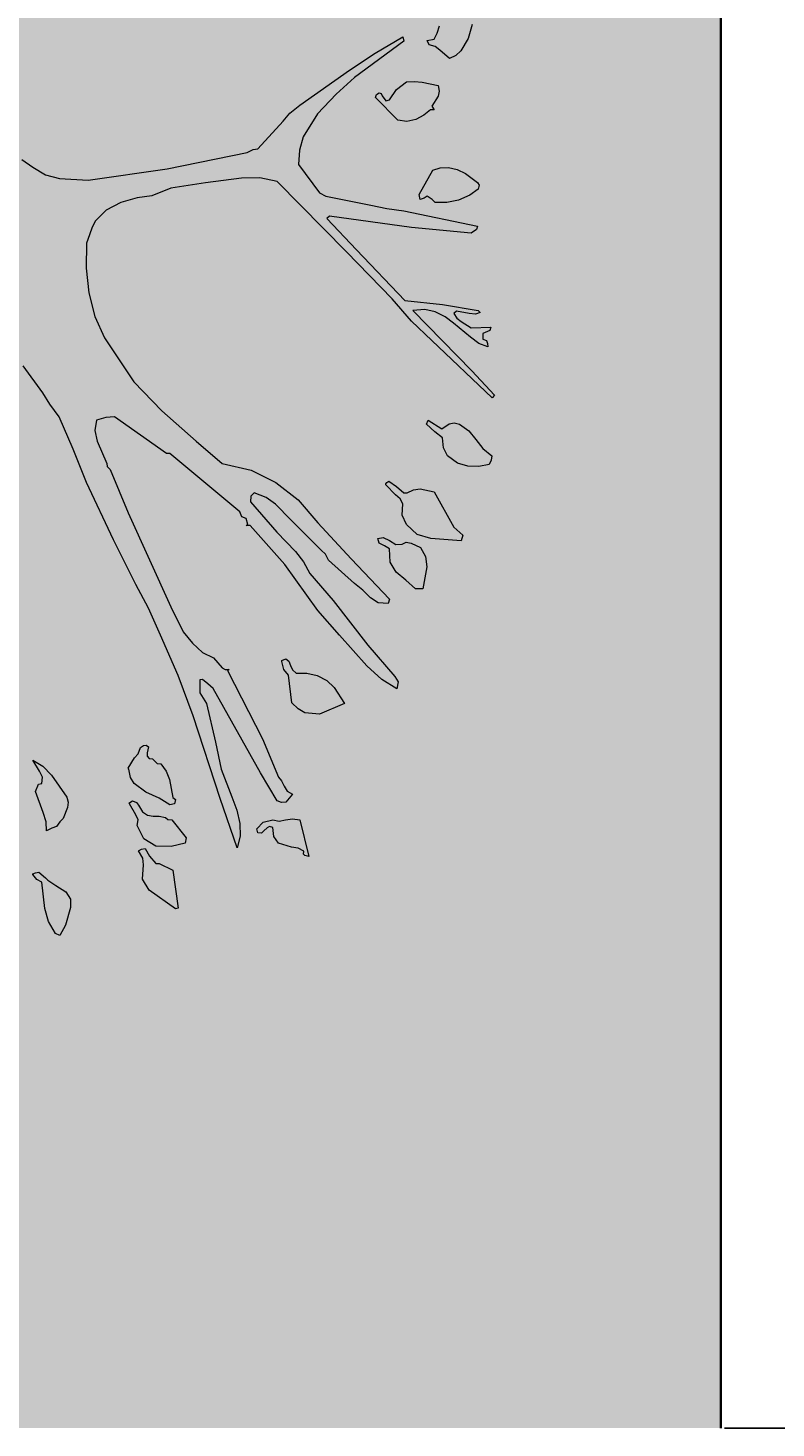
# Model space of a CAD drawing. Units: inches. Extents: x 84 to 1044, y -280 to 906.
# Tile 88 of 105: x 883 to 897, y 400 to 426. Entities that reach past the tile are written whole.
import ezdxf

# ---------------------------------------------------------------- set-up
doc = ezdxf.new("R2010")
doc.units = ezdxf.units.IN
for name, color, linetype, lineweight in [('A-ANNO-DIMS', 2, 'Continuous', 18), ('L-PLNT', 114, 'Continuous', 15), ('WALL', 250, 'Continuous', 35)]:
    doc.layers.add(name, color=color, linetype=linetype, lineweight=lineweight)
doc.layers.add('L-PLNT-PATT', color=9, linetype='Continuous', lineweight=9, true_color=0xafd9aa)
doc.styles.get("Standard").update_dxf_attribs({"font": 'arial.ttf'})
doc.dimstyles.get("Standard").update_dxf_attribs({"dimtxt": 0.18, "dimasz": 0.18, "dimexe": 0.18, "dimexo": 0.0625, "dimgap": 0.09, "dimtad": 0, "dimtih": 1, "dimtoh": 1, "dimdec": 4, "dimzin": 0, "dimdsep": 46, "dimtxsty": 'Standard', "dimcen": 0.09, "dimadec": 0, "dimazin": 0, "dimtfac": 1, "dimtdec": 4, "dimtofl": 0, "dimtmove": 0, "dimatfit": 3, "dimfxl": 1, "dimtolj": 1, "dimtzin": 0, "dimarcsym": 0})

# ---------------------------------------------------------------- blocks, each defined once
blk = doc.blocks.new('A$C37E508DF')
for p, q in [((1.3421, 1.0861), (1.3455, 1.0934)), ((1.3455, 1.0934), (1.3485, 1.102)), ((1.3875, 1.1037), (1.3828, 1.087)), ((1.3057, 1.0835), (1.2469, 1.0402)), ((1.2713, 1.0694), (1.3044, 1.0887)), ((1.3044, 1.0887), (1.3057, 1.0835)), ((1.3335, 1.0844), (1.3421, 1.0861)), ((1.3361, 1.0793), (1.3335, 1.0844)), ((1.3434, 1.0771), (1.3361, 1.0793)), ((1.349, 1.0728), (1.3434, 1.0771)), ((1.3605, 1.063), (1.349, 1.0728)), ((1.3828, 1.087), (1.3738, 1.072)), ((1.2409, 1.0488), (1.2713, 1.0694)), ((1.3678, 1.0664), (1.3605, 1.063)), ((1.3738, 1.072), (1.3678, 1.0664)), ((1.1813, 1.0072), (1.2409, 1.0488)), ((1.2469, 1.0402), (1.2246, 1.0201)), ((1.2885, 1.0136), (1.2971, 1.0257)), ((1.2971, 1.0257), (1.3091, 1.0351)), ((1.3091, 1.0351), (1.3185, 1.0355)), ((1.3185, 1.0355), (1.3275, 1.0347)), ((1.3275, 1.0347), (1.3468, 1.0308)), ((1.3468, 1.0308), (1.3481, 1.0239)), ((1.3481, 1.0239), (1.3468, 1.018)), ((1.1693, 0.9974), (1.1813, 1.0072)), ((1.2246, 1.0201), (1.2023, 0.9969)), ((1.2718, 1.0162), (1.2731, 1.0197)), ((1.2984, 0.9892), (1.2718, 1.0162)), ((1.2731, 1.0197), (1.2761, 1.0218)), ((1.2761, 1.0218), (1.2786, 1.0209)), ((1.2786, 1.0209), (1.2799, 1.0184)), ((1.2799, 1.0184), (1.2842, 1.0124)), ((1.2842, 1.0124), (1.2885, 1.0136)), ((1.3468, 1.018), (1.3391, 1.0059)), ((1.3391, 1.0059), (1.3421, 1.0016)), ((1.1612, 0.9879), (1.1693, 0.9974)), ((1.2023, 0.9969), (1.1852, 0.9691)), ((1.3095, 0.9875), (1.2984, 0.9892)), ((1.3202, 0.9901), (1.3095, 0.9875)), ((1.3297, 0.9952), (1.3202, 0.9901)), ((1.3378, 1.0016), (1.3297, 0.9952)), ((1.3421, 1.0016), (1.3378, 1.0016)), ((1.1311, 0.9549), (1.1612, 0.9879)), ((1.1256, 0.954), (1.1311, 0.9549)), ((1.1852, 0.9691), (1.1809, 0.9532)), ((0.8486, 0.942), (0.8619, 0.933)), ((1.0227, 0.9309), (1.1183, 0.9506)), ((1.1183, 0.9506), (1.1256, 0.954)), ((1.1809, 0.9532), (1.1796, 0.936)), ((0.8619, 0.933), (0.8769, 0.9236)), ((0.8769, 0.9236), (0.8936, 0.9193)), ((0.9279, 0.9172), (1.0227, 0.9309)), ((1.1796, 0.936), (1.2049, 0.9022)), ((1.3241, 0.9), (1.3404, 0.9292)), ((1.3404, 0.9292), (1.3494, 0.9322)), ((1.3494, 0.9322), (1.3592, 0.9326)), ((1.3592, 0.9326), (1.3695, 0.93)), ((1.3695, 0.93), (1.3794, 0.9253)), ((1.3794, 0.9253), (1.394, 0.9146)), ((0.8936, 0.9193), (0.9279, 0.9172)), ((1.0269, 0.9077), (1.0042, 0.8987)), ((1.0685, 0.9142), (1.0269, 0.9077)), ((1.1114, 0.9198), (1.0685, 0.9142)), ((1.1333, 0.9202), (1.1114, 0.9198)), ((1.1543, 0.9159), (1.1333, 0.9202)), ((1.2371, 0.8314), (1.1543, 0.9159)), ((1.3948, 0.9065), (1.3846, 0.8992)), ((1.394, 0.9146), (1.3957, 0.9112)), ((1.3957, 0.9112), (1.3948, 0.9065)), ((0.9673, 0.8906), (0.9498, 0.8816)), ((0.9866, 0.8962), (0.9673, 0.8906)), ((1.0042, 0.8987), (0.9866, 0.8962)), ((1.2049, 0.9022), (1.2126, 0.8983)), ((1.2126, 0.8983), (1.2662, 0.8876)), ((1.3254, 0.8944), (1.3241, 0.9)), ((1.3301, 0.8957), (1.3254, 0.8944)), ((1.3335, 0.8983), (1.3301, 0.8957)), ((1.3395, 0.8944), (1.3335, 0.8983)), ((1.3434, 0.8906), (1.3395, 0.8944)), ((1.3571, 0.8906), (1.3434, 0.8906)), ((1.3713, 0.8936), (1.3571, 0.8906)), ((1.3846, 0.8992), (1.3713, 0.8936)), ((0.9498, 0.8816), (0.9369, 0.8687)), ((1.2169, 0.8743), (1.2135, 0.8713)), ((1.2135, 0.8713), (1.2491, 0.834)), ((1.3151, 0.8606), (1.2169, 0.8743)), ((1.2662, 0.8876), (1.2855, 0.8833)), ((1.2855, 0.8833), (1.3057, 0.8807)), ((1.3057, 0.8807), (1.394, 0.8623)), ((0.933, 0.861), (0.9296, 0.852)), ((0.9369, 0.8687), (0.933, 0.861)), ((1.3863, 0.8541), (1.3151, 0.8606)), ((1.3927, 0.8584), (1.3863, 0.8541)), ((1.394, 0.8623), (1.3927, 0.8584)), ((0.9262, 0.8421), (0.9257, 0.8121)), ((0.9296, 0.852), (0.9262, 0.8421)), ((1.2919, 0.7752), (1.2371, 0.8314)), ((1.2491, 0.834), (1.3069, 0.7735)), ((0.9257, 0.8121), (0.9287, 0.7825)), ((0.9287, 0.7825), (0.936, 0.7542)), ((1.3151, 0.7487), (1.2919, 0.7752)), ((1.3069, 0.7735), (1.352, 0.7684)), ((0.936, 0.7542), (0.9476, 0.7285)), ((1.3309, 0.7624), (1.3164, 0.7615)), ((1.3164, 0.7615), (1.3871, 0.6891)), ((1.3434, 0.7598), (1.3309, 0.7624)), ((1.355, 0.7538), (1.3434, 0.7598)), ((1.352, 0.7684), (1.3948, 0.7615)), ((1.3653, 0.7461), (1.355, 0.7538)), ((1.3687, 0.7607), (1.3657, 0.7577)), ((1.3657, 0.7577), (1.3691, 0.7521)), ((1.3841, 0.7577), (1.3687, 0.7607)), ((1.3914, 0.7572), (1.3841, 0.7577)), ((1.397, 0.759), (1.3914, 0.7572)), ((1.3948, 0.7615), (1.397, 0.759)), ((1.3391, 0.7255), (1.3151, 0.7487)), ((1.3854, 0.7294), (1.3653, 0.7461)), ((1.3691, 0.7521), (1.3743, 0.7482)), ((1.3743, 0.7482), (1.3863, 0.7405)), ((1.3863, 0.7405), (1.4099, 0.7414)), ((1.4086, 0.7375), (1.4004, 0.7337)), ((1.4099, 0.7414), (1.4086, 0.7375)), ((0.9476, 0.7285), (0.9828, 0.6762)), ((1.4116, 0.6569), (1.3391, 0.7255)), ((1.3953, 0.7221), (1.3854, 0.7294)), ((1.4064, 0.7178), (1.3953, 0.7221)), ((1.4004, 0.7337), (1.4004, 0.7272)), ((1.4004, 0.7272), (1.4047, 0.7255)), ((1.4047, 0.7255), (1.406, 0.7221)), ((1.406, 0.7221), (1.4064, 0.7178)), ((0.8739, 0.6629), (0.8503, 0.6951)), ((1.3871, 0.6891), (1.4141, 0.6599)), ((0.9828, 0.6762), (1.0162, 0.6415)), ((0.8824, 0.6492), (0.8739, 0.6629)), ((1.4141, 0.6599), (1.4116, 0.6569)), ((0.8932, 0.6342), (0.8824, 0.6492)), ((1.0162, 0.6415), (1.0574, 0.605)), ((0.9103, 0.5956), (0.8932, 0.6342)), ((0.9382, 0.6303), (0.936, 0.6179)), ((0.9493, 0.6333), (0.9382, 0.6303)), ((0.9596, 0.6342), (0.9493, 0.6333)), ((1.0218, 0.5904), (0.9596, 0.6342)), ((1.3327, 0.6252), (1.3348, 0.6303)), ((1.343, 0.6162), (1.3327, 0.6252)), ((1.3348, 0.6303), (1.3511, 0.62)), ((1.3511, 0.62), (1.3601, 0.6256)), ((1.3601, 0.6256), (1.3661, 0.6269)), ((1.3661, 0.6269), (1.3725, 0.6252)), ((1.3725, 0.6252), (1.3837, 0.6175)), ((0.936, 0.6179), (0.939, 0.605)), ((0.939, 0.605), (0.9506, 0.5784)), ((1.0574, 0.605), (1.0883, 0.5784)), ((1.352, 0.6089), (1.343, 0.6162)), ((1.3533, 0.5969), (1.352, 0.6089)), ((1.3837, 0.6175), (1.3918, 0.6072)), ((1.3918, 0.6072), (1.4004, 0.5964)), ((0.9262, 0.5557), (0.9103, 0.5956)), ((1.0256, 0.5904), (1.0218, 0.5904)), ((1.1097, 0.5205), (1.0256, 0.5904)), ((1.358, 0.5874), (1.3533, 0.5969)), ((1.37, 0.5789), (1.358, 0.5874)), ((1.4004, 0.5964), (1.4111, 0.5874)), ((1.4111, 0.5874), (1.4103, 0.5823)), ((0.9506, 0.5784), (0.951, 0.5746)), ((0.951, 0.5746), (0.9545, 0.5711)), ((0.9545, 0.5711), (0.9759, 0.5193)), ((1.0883, 0.5784), (1.123, 0.5703)), ((1.123, 0.5703), (1.1526, 0.5557)), ((1.3824, 0.575), (1.37, 0.5789)), ((1.3953, 0.5746), (1.3824, 0.575)), ((1.4077, 0.5771), (1.3953, 0.5746)), ((1.4103, 0.5823), (1.4077, 0.5771)), ((0.9583, 0.4871), (0.9262, 0.5557)), ((1.1526, 0.5557), (1.1792, 0.5347)), ((1.2842, 0.554), (1.2855, 0.5557)), ((1.2842, 0.5527), (1.2842, 0.554)), ((1.2855, 0.5557), (1.2876, 0.557)), ((1.2876, 0.557), (1.2971, 0.551)), ((1.1226, 0.5394), (1.1221, 0.5325)), ((1.1268, 0.5433), (1.1226, 0.5394)), ((1.141, 0.5377), (1.1268, 0.5433)), ((1.1521, 0.5296), (1.141, 0.5377)), ((1.2958, 0.5407), (1.2842, 0.5527)), ((1.3014, 0.536), (1.2958, 0.5407)), ((1.2971, 0.551), (1.3057, 0.5433)), ((1.3057, 0.5433), (1.3099, 0.5433)), ((1.3099, 0.5433), (1.3172, 0.5467)), ((1.3172, 0.5467), (1.3254, 0.548)), ((1.3254, 0.548), (1.3421, 0.5446)), ((1.3421, 0.5446), (1.3657, 0.5021)), ((1.1118, 0.5145), (1.1097, 0.5205)), ((1.1221, 0.5325), (1.1539, 0.4961)), ((1.1706, 0.5111), (1.1521, 0.5296)), ((1.1792, 0.5347), (1.2027, 0.5072)), ((1.3044, 0.53), (1.3014, 0.536)), ((1.3039, 0.5167), (1.3044, 0.53)), ((0.9759, 0.5193), (1.0269, 0.4069)), ((1.117, 0.5124), (1.1118, 0.5145)), ((1.1191, 0.5055), (1.117, 0.5124)), ((1.117, 0.5042), (1.1191, 0.5055)), ((1.1217, 0.5042), (1.117, 0.5042)), ((1.1633, 0.4575), (1.1217, 0.5042)), ((1.1955, 0.4858), (1.1706, 0.5111)), ((1.2027, 0.5072), (1.2426, 0.4644)), ((1.3091, 0.5055), (1.3039, 0.5167)), ((1.3215, 0.4935), (1.3091, 0.5055)), ((0.9853, 0.4335), (0.9583, 0.4871)), ((1.1539, 0.4961), (1.1762, 0.4729)), ((1.207, 0.4747), (1.1955, 0.4858)), ((1.2748, 0.4884), (1.2812, 0.4897)), ((1.2761, 0.4832), (1.2748, 0.4884)), ((1.2812, 0.4897), (1.2885, 0.4862)), ((1.2885, 0.4862), (1.2962, 0.4815)), ((1.3382, 0.4884), (1.3215, 0.4935)), ((1.3743, 0.4858), (1.3382, 0.4884)), ((1.3657, 0.5021), (1.3764, 0.4927)), ((1.3764, 0.4927), (1.3743, 0.4858)), ((1.1762, 0.4729), (1.1856, 0.4605)), ((1.2122, 0.47), (1.207, 0.4747)), ((1.2156, 0.4627), (1.2122, 0.47)), ((1.2825, 0.4798), (1.2761, 0.4832)), ((1.2885, 0.4764), (1.2825, 0.4798)), ((1.2894, 0.4601), (1.2885, 0.4764)), ((1.2962, 0.4815), (1.3039, 0.482)), ((1.3039, 0.482), (1.3087, 0.4841)), ((1.3087, 0.4841), (1.3147, 0.4832)), ((1.3147, 0.4832), (1.3258, 0.4777)), ((1.3258, 0.4777), (1.3318, 0.4669)), ((1.2027, 0.4026), (1.1633, 0.4575)), ((1.1856, 0.4605), (1.1933, 0.4468)), ((1.2469, 0.4348), (1.2156, 0.4627)), ((1.2426, 0.4644), (1.2885, 0.4159)), ((1.2967, 0.4485), (1.2894, 0.4601)), ((1.3331, 0.4545), (1.3284, 0.4284)), ((1.3318, 0.4669), (1.3331, 0.4545)), ((1.1933, 0.4468), (1.2212, 0.4146)), ((1.3082, 0.4386), (1.2967, 0.4485)), ((1.3198, 0.4284), (1.3082, 0.4386)), ((1.0003, 0.4052), (0.9853, 0.4335)), ((1.2568, 0.4266), (1.2469, 0.4348)), ((1.2658, 0.4176), (1.2568, 0.4266)), ((1.3284, 0.4284), (1.3198, 0.4284)), ((1.0145, 0.373), (1.0003, 0.4052)), ((1.0269, 0.4069), (1.0419, 0.3769)), ((1.2289, 0.373), (1.2027, 0.4026)), ((1.2212, 0.4146), (1.2628, 0.361)), ((1.2752, 0.4116), (1.2658, 0.4176)), ((1.2868, 0.4108), (1.2752, 0.4116)), ((1.2885, 0.4159), (1.2868, 0.4108)), ((1.0359, 0.3246), (1.0145, 0.373)), ((1.0419, 0.3769), (1.0527, 0.3632)), ((1.2615, 0.3362), (1.2289, 0.373)), ((1.0527, 0.3632), (1.0647, 0.352)), ((1.0647, 0.352), (1.078, 0.346)), ((1.2628, 0.361), (1.2949, 0.3233)), ((1.078, 0.346), (1.0883, 0.334)), ((1.1599, 0.3426), (1.1646, 0.3447)), ((1.1599, 0.3413), (1.1599, 0.3426)), ((1.162, 0.3319), (1.1599, 0.3413)), ((1.1646, 0.3447), (1.168, 0.3417)), ((1.168, 0.3417), (1.1702, 0.3366)), ((1.1702, 0.3366), (1.1727, 0.3314)), ((1.2795, 0.3199), (1.2615, 0.3362)), ((1.0535, 0.2766), (1.0359, 0.3246)), ((1.0647, 0.3199), (1.0617, 0.3194)), ((1.0617, 0.3194), (1.0617, 0.304)), ((1.0711, 0.3147), (1.0647, 0.3199)), ((1.0883, 0.334), (1.0921, 0.3319)), ((1.0921, 0.3319), (1.0968, 0.3319)), ((1.0968, 0.3319), (1.0947, 0.3306)), ((1.0947, 0.3306), (1.1367, 0.2491)), ((1.1676, 0.325), (1.162, 0.3319)), ((1.1719, 0.292), (1.1676, 0.325)), ((1.1727, 0.3314), (1.177, 0.3276)), ((1.177, 0.3276), (1.1895, 0.3276)), ((1.1895, 0.3276), (1.2019, 0.3246)), ((1.2019, 0.3246), (1.2135, 0.3186)), ((1.2135, 0.3186), (1.2225, 0.3104)), ((1.2975, 0.3087), (1.2795, 0.3199)), ((1.2949, 0.3233), (1.2988, 0.3173)), ((1.0617, 0.304), (1.0698, 0.2911)), ((1.0775, 0.3092), (1.0711, 0.3147)), ((1.1341, 0.2084), (1.0775, 0.3092)), ((1.2225, 0.3104), (1.2349, 0.2911)), ((1.2988, 0.3173), (1.2975, 0.3087)), ((1.0698, 0.2911), (1.0805, 0.2448)), ((1.1792, 0.2847), (1.1719, 0.292)), ((1.2349, 0.2911), (1.2049, 0.2783)), ((1.0861, 0.1775), (1.0535, 0.2766)), ((1.1873, 0.28), (1.1792, 0.2847)), ((1.2049, 0.2783), (1.1873, 0.28)), ((0.9879, 0.2311), (0.9905, 0.2384)), ((0.9905, 0.2384), (0.9943, 0.241)), ((0.9943, 0.241), (0.9973, 0.2414)), ((0.9973, 0.2414), (1.0003, 0.2393)), ((1.0003, 0.2393), (0.9986, 0.232)), ((1.0805, 0.2448), (1.087, 0.2127)), ((1.1367, 0.2491), (1.1556, 0.2032)), ((0.8619, 0.2234), (0.8739, 0.2161)), ((0.87, 0.2101), (0.8619, 0.2234)), ((0.9759, 0.214), (0.9836, 0.226)), ((0.9836, 0.226), (0.9879, 0.2311)), ((0.9986, 0.232), (0.9986, 0.2281)), ((0.9986, 0.2281), (1.0012, 0.2255)), ((1.0012, 0.2255), (1.0051, 0.2251)), ((1.0051, 0.2251), (1.0076, 0.2225)), ((1.0076, 0.2225), (1.0106, 0.2195)), ((1.0106, 0.2195), (1.0149, 0.2191)), ((1.0149, 0.2191), (1.0214, 0.2101)), ((0.8734, 0.2032), (0.87, 0.2101)), ((0.8726, 0.1955), (0.8734, 0.2032)), ((0.8739, 0.2161), (0.8841, 0.2054)), ((0.8841, 0.2054), (0.9026, 0.1792)), ((0.9768, 0.2127), (0.9759, 0.214)), ((0.9789, 0.2028), (0.9768, 0.2127)), ((0.9832, 0.1955), (0.9789, 0.2028)), ((1.0214, 0.2101), (1.0252, 0.2002)), ((1.087, 0.2127), (1.0998, 0.1797)), ((1.1543, 0.1749), (1.1341, 0.2084)), ((1.1556, 0.2032), (1.1594, 0.1985)), ((0.8649, 0.1857), (0.8687, 0.1947)), ((0.8743, 0.1608), (0.8649, 0.1857)), ((0.8687, 0.1947), (0.8726, 0.1955)), ((0.9969, 0.1852), (0.9832, 0.1955)), ((1.0132, 0.1779), (0.9969, 0.1852)), ((1.0252, 0.2002), (1.0295, 0.1788)), ((1.1594, 0.1985), (1.1624, 0.1921)), ((1.1624, 0.1921), (1.1663, 0.1861)), ((1.1663, 0.1861), (1.1727, 0.1827)), ((0.9026, 0.1792), (0.9043, 0.1732)), ((0.9043, 0.1732), (0.9035, 0.1668)), ((0.9768, 0.1719), (0.9811, 0.1749)), ((0.9776, 0.1711), (0.9768, 0.1719)), ((0.9853, 0.1578), (0.9776, 0.1711)), ((0.9811, 0.1749), (0.9858, 0.1728)), ((0.9858, 0.1728), (0.9884, 0.1694)), ((0.9884, 0.1694), (0.9931, 0.1616)), ((1.0256, 0.1698), (1.0132, 0.1779)), ((1.0312, 0.1711), (1.0256, 0.1698)), ((1.0295, 0.1788), (1.0325, 0.1762)), ((1.0325, 0.1762), (1.0312, 0.1711)), ((1.1063, 0.1183), (1.0861, 0.1775)), ((1.0998, 0.1797), (1.1058, 0.1634)), ((1.1594, 0.1728), (1.1543, 0.1749)), ((1.1646, 0.1732), (1.1594, 0.1728)), ((1.1727, 0.1827), (1.1646, 0.1732)), ((0.8777, 0.1496), (0.8743, 0.1608)), ((0.8983, 0.1535), (0.894, 0.1496)), ((0.9035, 0.1668), (0.8983, 0.1535)), ((0.9879, 0.1518), (0.9853, 0.1578)), ((0.9866, 0.1453), (0.9879, 0.1518)), ((0.9931, 0.1616), (0.9991, 0.1574)), ((0.9991, 0.1574), (1.0059, 0.1565)), ((1.0059, 0.1565), (1.0132, 0.1565)), ((1.0132, 0.1565), (1.0205, 0.1548)), ((1.0205, 0.1548), (1.0235, 0.1522)), ((1.0235, 0.1522), (1.0282, 0.1518)), ((1.0282, 0.1518), (1.0454, 0.1303)), ((1.1058, 0.1634), (1.1097, 0.1475)), ((1.1376, 0.1492), (1.1491, 0.1518)), ((1.1491, 0.1518), (1.1564, 0.1505)), ((1.1564, 0.1505), (1.1642, 0.1518)), ((1.1642, 0.1518), (1.1727, 0.1531)), ((1.1727, 0.1531), (1.1813, 0.1518)), ((1.1813, 0.1518), (1.192, 0.108)), ((0.8781, 0.1389), (0.8777, 0.1496)), ((0.8846, 0.1419), (0.8781, 0.1389)), ((0.8902, 0.1441), (0.8846, 0.1419)), ((0.894, 0.1496), (0.8902, 0.1441)), ((0.9948, 0.1291), (0.9866, 0.1453)), ((1.1097, 0.1475), (1.1101, 0.1325)), ((1.1298, 0.1411), (1.1376, 0.1492)), ((1.1311, 0.1364), (1.1298, 0.1411)), ((1.1354, 0.1359), (1.1311, 0.1364)), ((1.1384, 0.1389), (1.1354, 0.1359)), ((1.1423, 0.1423), (1.1384, 0.1389)), ((1.1449, 0.1441), (1.1423, 0.1423)), ((1.1491, 0.1428), (1.1449, 0.1441)), ((1.1504, 0.132), (1.1491, 0.1428)), ((0.9918, 0.117), (0.9961, 0.1175)), ((1.0089, 0.1205), (0.9948, 0.1291)), ((0.9961, 0.1175), (1.0016, 0.1085)), ((1.0274, 0.12), (1.0089, 0.1205)), ((1.0441, 0.1239), (1.0274, 0.12)), ((1.0454, 0.1303), (1.0441, 0.1239)), ((1.1101, 0.1325), (1.1063, 0.1183)), ((1.1556, 0.1239), (1.1504, 0.132)), ((1.1714, 0.1192), (1.1556, 0.1239)), ((1.1792, 0.1179), (1.1714, 0.1192)), ((1.186, 0.1145), (1.1792, 0.1179)), ((0.9884, 0.1149), (0.9918, 0.117)), ((0.9935, 0.1063), (0.9884, 0.1149)), ((0.9943, 0.0982), (0.9935, 0.1063)), ((1.0016, 0.1085), (1.0089, 0.0999)), ((1.1856, 0.111), (1.186, 0.1145)), ((1.1873, 0.1093), (1.1856, 0.111)), ((1.192, 0.108), (1.1873, 0.1093)), ((0.8619, 0.0875), (0.8649, 0.0887)), ((0.8619, 0.0866), (0.8619, 0.0875)), ((0.8666, 0.0806), (0.8619, 0.0866)), ((0.8649, 0.0887), (0.8691, 0.0892)), ((0.8691, 0.0892), (0.8769, 0.0827)), ((0.9931, 0.081), (0.9943, 0.0982)), ((1.0089, 0.0999), (1.0132, 0.0999)), ((1.0132, 0.0999), (1.0295, 0.0917)), ((1.0295, 0.0917), (1.0359, 0.0463)), ((0.8726, 0.0776), (0.8666, 0.0806)), ((0.8764, 0.0459), (0.8726, 0.0776)), ((0.8769, 0.0827), (0.8799, 0.0797)), ((0.8799, 0.0797), (0.8893, 0.0733)), ((0.8893, 0.0733), (0.9013, 0.066)), ((1.0012, 0.0677), (0.9931, 0.081)), ((1.0325, 0.0454), (1.0012, 0.0677)), ((0.9013, 0.066), (0.9069, 0.057)), ((0.9069, 0.057), (0.9069, 0.0471)), ((0.8807, 0.0304), (0.8764, 0.0459)), ((0.9069, 0.0471), (0.9009, 0.0261)), ((1.0359, 0.0463), (1.0325, 0.0454)), ((0.8889, 0.0159), (0.8807, 0.0304)), ((0.9009, 0.0261), (0.894, 0.0137)), ((0.894, 0.0137), (0.8889, 0.0159))]:
    blk.add_line(p, q)
blk = doc.blocks.new('*D62')
at = {"layer": 'A-ANNO-DIMS', "color": 0, "lineweight": -2, "transparency": 16777216}
for p, q in [((203.179, 709.183), (203.179, 905.9)), ((203.359, 905.72), (549.232, 905.72)), ((895.894, 905.72), (550.021, 905.72)), ((896.074, 400.183), (896.074, 905.9))]:
    blk.add_line(p, q, dxfattribs=at)
at = {"layer": 'A-ANNO-DIMS', "color": 0, "transparency": 16777216}
for points in [[(203.359, 905.75), (203.359, 905.69), (203.179, 905.72)], [(895.894, 905.75), (895.894, 905.69), (896.074, 905.72)]]:
    blk.add_solid(points, dxfattribs=at)
at = {"layer": 'Defpoints', "color": 0, "transparency": 16777216}
for p in [(896.074, 905.72), (203.179, 709.12), (896.074, 400.12)]:
    blk.add_point(p, dxfattribs=at)
at = {"layer": 'A-ANNO-DIMS', "color": 0, "transparency": 16777216, "insert": (549.627, 905.72), "char_height": 0.18, "attachment_point": 5}
blk.add_mtext('\\A1;692.9', dxfattribs=at)
blk = doc.blocks.new('*D63')
at = {"layer": 'A-ANNO-DIMS', "color": 0, "lineweight": -2, "transparency": 16777216}
for p, q in [((833.136, 709.12), (1043.768, 709.12)), ((1043.588, 708.94), (1043.588, 400.302)), ((1043.588, 91.3), (1043.588, 399.938)), ((896.136, 91.12), (1043.768, 91.12))]:
    blk.add_line(p, q, dxfattribs=at)
at = {"layer": 'A-ANNO-DIMS', "color": 0, "transparency": 16777216}
for points in [[(1043.558, 708.94), (1043.618, 708.94), (1043.588, 709.12)], [(1043.558, 91.3), (1043.618, 91.3), (1043.588, 91.12)]]:
    blk.add_solid(points, dxfattribs=at)
at = {"layer": 'Defpoints', "color": 0, "transparency": 16777216}
for p in [(833.074, 709.12), (1043.588, 709.12), (896.074, 91.12)]:
    blk.add_point(p, dxfattribs=at)
at = {"layer": 'A-ANNO-DIMS', "color": 0, "transparency": 16777216, "insert": (1043.588, 400.12), "char_height": 0.18, "attachment_point": 5}
blk.add_mtext('\\A1;618', dxfattribs=at)
blk = doc.blocks.new('*D65')
at = {"layer": 'A-ANNO-DIMS', "color": 0, "lineweight": -2, "transparency": 16777216}
for p, q in [((896.074, 400.183), (896.074, 905.9)), ((896.254, 905.72), (943.855, 905.72)), ((991.894, 905.72), (944.293, 905.72)), ((992.074, 856.183), (992.074, 905.9))]:
    blk.add_line(p, q, dxfattribs=at)
at = {"layer": 'A-ANNO-DIMS', "color": 0, "transparency": 16777216}
for points in [[(896.254, 905.75), (896.254, 905.69), (896.074, 905.72)], [(991.894, 905.75), (991.894, 905.69), (992.074, 905.72)]]:
    blk.add_solid(points, dxfattribs=at)
at = {"layer": 'Defpoints', "color": 0, "transparency": 16777216}
for p in [(896.074, 905.72), (992.074, 856.12), (896.074, 400.12)]:
    blk.add_point(p, dxfattribs=at)
at = {"layer": 'A-ANNO-DIMS', "color": 0, "transparency": 16777216, "insert": (944.074, 905.72), "char_height": 0.18, "attachment_point": 5}
blk.add_mtext('\\A1;96', dxfattribs=at)
blk = doc.blocks.new('*D76')
at = {"layer": 'A-ANNO-DIMS', "color": 0, "lineweight": -2, "transparency": 16777216}
for p, q in [((896.136, 400.12), (1043.768, 400.12)), ((1043.588, 399.94), (1043.588, 391.302)), ((1043.588, 382.3), (1043.588, 390.938)), ((896.136, 382.12), (1043.768, 382.12))]:
    blk.add_line(p, q, dxfattribs=at)
at = {"layer": 'A-ANNO-DIMS', "color": 0, "transparency": 16777216}
for points in [[(1043.558, 399.94), (1043.618, 399.94), (1043.588, 400.12)], [(1043.558, 382.3), (1043.618, 382.3), (1043.588, 382.12)]]:
    blk.add_solid(points, dxfattribs=at)
at = {"layer": 'Defpoints', "color": 0, "transparency": 16777216}
for p in [(896.074, 400.12), (1043.588, 400.12), (896.074, 382.12)]:
    blk.add_point(p, dxfattribs=at)
at = {"layer": 'A-ANNO-DIMS', "color": 0, "transparency": 16777216, "insert": (1043.588, 391.12), "char_height": 0.18, "attachment_point": 5}
blk.add_mtext('\\A1;18', dxfattribs=at)

msp = doc.modelspace()

# ---------------------------------------------------------------- hatches: boundary and pattern name
at = {"layer": 'L-PLNT-PATT', "transparency": 33554597}
h = msp.add_hatch(color=256, dxfattribs=at)
h.dxf.hatch_style = 1
h.paths.add_polyline_path([(896.074, 511.12), (704.074, 511.12), (704.074, 491.62), (704.074, 419.62), (704.074, 400.12), (833.074, 400.12), (896.074, 400.12)])

# ---------------------------------------------------------------- linework, layer by layer
at = {"layer": 'WALL'}
msp.add_line((896.074, 400.12), (896.074, 511.12), dxfattribs=at)

# ---------------------------------------------------------------- block references
at = {"layer": 'L-PLNT', "xscale": 15.19586232982809, "yscale": 15.19586232982809, "zscale": 15.19586232982809}
msp.add_blockref('A$C37E508DF', (870.466, 408.868), dxfattribs=at)

# ---------------------------------------------------------------- dimensions: what is measured, and where the dimension line sits
at = {"layer": 'A-ANNO-DIMS'}
for p1, override, picture, middle in [((203.179, 709.12), {"dimdec": 1, "dimlfac": 1, "dimrnd": 0, "dimzin": 0, "dimdsep": 46, "dimlunit": 2}, '*D62', (549.627, 905.72)), ((992.074, 856.12), {"dimdec": 0, "dimlfac": 1, "dimrnd": 0, "dimzin": 0, "dimdsep": 46, "dimlunit": 2}, '*D65', (944.074, 905.72))]:
    dim = msp.add_linear_dim(base=(896.074, 905.72), p1=p1, p2=(896.074, 400.12), dimstyle='Standard', override=override, dxfattribs=at)
    dim.commit()
    dim.dimension.update_dxf_attribs({"geometry": picture, "text_midpoint": middle})
for base, p1, p2, picture, middle in [((1043.588, 709.12), (896.074, 91.12), (833.074, 709.12), '*D63', (1043.588, 400.12)), ((1043.588, 400.12), (896.074, 382.12), (896.074, 400.12), '*D76', (1043.588, 391.12))]:
    dim = msp.add_linear_dim(base=base, p1=p1, p2=p2, angle=90, dimstyle='Standard', override={"dimdec": 0, "dimlfac": 1, "dimrnd": 0, "dimzin": 0, "dimdsep": 46, "dimlunit": 2}, dxfattribs=at)
    dim.commit()
    dim.dimension.update_dxf_attribs({"geometry": picture, "text_midpoint": middle})

doc.saveas('drawing.dxf')
